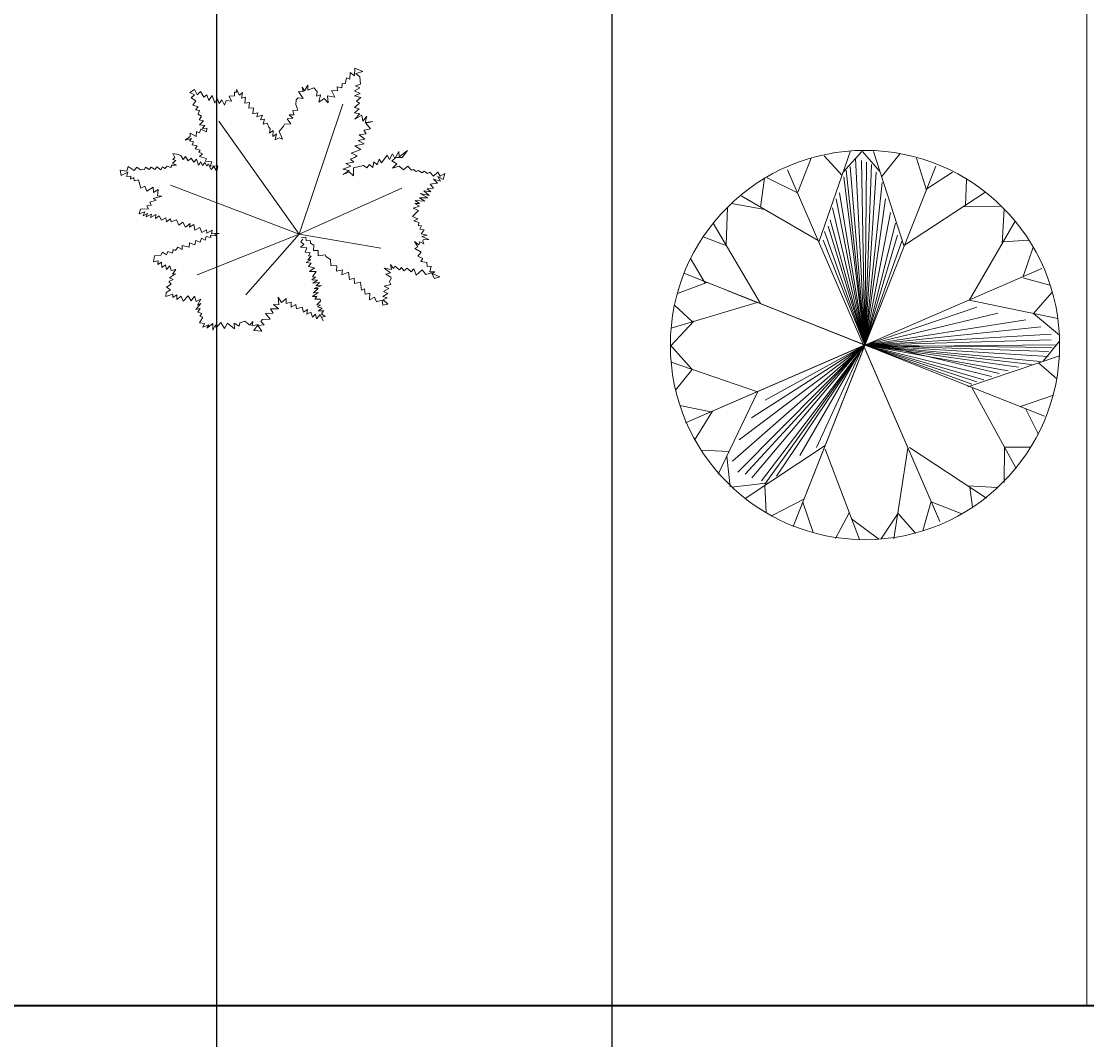
# Model space of a CAD drawing. Units: inches. Extents: x 8049 to 8459, y 820 to 1350.
# Tile 13 of 25: x 8170 to 8197, y 853 to 879. Entities that reach past the tile are written whole.
import ezdxf

# ---------------------------------------------------------------- set-up
doc = ezdxf.new("R2010")
doc.units = ezdxf.units.IN
doc.header["$MEASUREMENT"] = 0
for name, color, linetype, lineweight in [('A-ANNO-DIMS', 2, 'Continuous', 18), ('C-SITE-WALL', 7, 'Continuous', 35), ('L-PLNT-BEDS', 94, 'Continuous', 18), ('zelen', 69, 'Continuous', 13)]:
    doc.layers.add(name, color=color, linetype=linetype, lineweight=lineweight)
doc.styles.get("Standard").update_dxf_attribs({"font": 'arial.ttf'})
doc.dimstyles.get("Standard").update_dxf_attribs({"dimtxt": 0.18, "dimasz": 0.18, "dimexe": 0.18, "dimexo": 0.0625, "dimgap": 0.09, "dimtad": 0, "dimtih": 1, "dimtoh": 1, "dimdec": 4, "dimzin": 0, "dimdsep": 46, "dimtxsty": 'Standard', "dimcen": 0.09, "dimadec": 0, "dimazin": 0, "dimtfac": 1, "dimtdec": 4, "dimtofl": 0, "dimtmove": 0, "dimatfit": 3, "dimfxl": 1, "dimtolj": 1, "dimtzin": 0, "dimarcsym": 0})

# ---------------------------------------------------------------- blocks, each defined once
blk = doc.blocks.new('z_85')
for p, q in [((154.8, 474.2), (155.6, 493.8)), ((155.6, 493.8), (168.5, 483.9)), ((168.5, 483.9), (169.7, 507.5)), ((169.7, 507.5), (194.7, 497.5)), ((194.7, 497.5), (173, 491.4)), ((173, 491.4), (185.2, 481.2)), ((130, 447.6), (130.9, 460.7)), ((130.9, 460.7), (140.4, 459.9)), ((140.4, 459.9), (144.1, 478.3)), ((144.1, 478.3), (154.8, 474.2)), ((186.9, 458.5), (172.1, 453.2)), ((185.2, 481.2), (186.9, 458.5)), ((-334.5, 433), (-320.5, 441.8)), ((-320.3, 426.3), (-334.5, 433)), ((-331, 417), (-320.3, 426.3)), ((-320.5, 441.8), (-312.2, 426.3)), ((-312.2, 426.3), (-302, 436.4)), ((-302, 436.4), (-292.5, 418.9)), ((-292.5, 418.9), (-282.7, 426.1)), ((-282.7, 426.1), (-277, 408.1)), ((-198.5, 423), (-198.2, 434.1)), ((-198.2, 434.1), (-192.6, 433.8)), ((-192.6, 433.8), (-192.5, 442.2)), ((-192.5, 442.2), (-183.3, 424.5)), ((-183.3, 424.5), (-173.3, 433.2)), ((-173.3, 433.2), (-176.4, 415.5)), ((-2.1, 435.8), (11.7, 434.9)), ((11.4, 414.5), (-2.1, 435.8)), ((8.4, 449), (15.4, 438)), ((11.7, 434.9), (8.4, 449)), ((15.4, 438), (25.6, 455.6)), ((25.6, 455.6), (26.4, 439.7)), ((26.4, 439.7), (44.1, 447.4)), ((44.1, 447.4), (54.4, 436.3)), ((54.4, 436.3), (52.3, 421.7)), ((52.3, 421.7), (64.6, 426)), ((64.6, 426), (59.8, 403.9)), ((98.5, 438.8), (116.6, 438)), ((108.9, 418.4), (98.5, 438.8)), ((116.1, 450.2), (130, 447.6)), ((116.6, 438), (116.1, 450.2)), ((185.1, 447.3), (169, 438)), ((169, 438), (186.4, 430.3)), ((186.4, 430.3), (169.1, 422.7)), ((172.1, 453.2), (185.1, 447.3)), ((-316.9, 407.2), (-331, 417)), ((-325.3, 394.5), (-316.9, 407.2)), ((-309.5, 388.7), (-325.3, 394.5)), ((-277, 408.1), (-266.3, 423.5)), ((-266.3, 423.5), (-258.7, 400.7)), ((-258.7, 400.7), (-250.8, 414.2)), ((-250.8, 414.2), (-244.9, 399.8)), ((-244.9, 399.8), (-237.2, 410.8)), ((-237.2, 410.8), (-228.5, 393.9)), ((-228.5, 393.9), (-223.5, 408.6)), ((-223.5, 408.6), (-207.8, 406.4)), ((-214.2, 421.3), (-198.5, 423)), ((-207.8, 406.4), (-214.2, 421.3)), ((-176.4, 415.5), (-165.1, 418.9)), ((-165.1, 418.9), (-166.4, 400.3)), ((-166.4, 400.3), (-152.4, 402.8)), ((-152.4, 402.8), (-154.8, 385.2)), ((-10.8, 396), (-9.6, 410.9)), ((-4.1, 379.1), (-10.8, 396)), ((-9.6, 410.9), (-3.8, 416.9)), ((-3.8, 416.9), (11.4, 414.5)), ((0, 0), (132.7, 397)), ((59.8, 403.9), (75.6, 414.2)), ((75.6, 414.2), (88.3, 401.4)), ((86.4, 422.5), (108.9, 418.4)), ((88.3, 401.4), (86.4, 422.5)), ((169.1, 422.7), (188.1, 417.5)), ((183.6, 400.7), (169.1, 387.1)), ((188.1, 417.5), (174.5, 406.5)), ((174.5, 406.5), (183.6, 400.7)), ((-317.2, 380.4), (-309.5, 388.7)), ((-305.1, 378.2), (-317.2, 380.4)), ((-309.5, 366.8), (-305.1, 378.2)), ((-299.2, 360.3), (-309.5, 366.8)), ((-305.9, 349.8), (-299.2, 360.3)), ((-154.8, 385.2), (-139.8, 385.6)), ((-139.8, 385.6), (-142, 367.5)), ((-142, 367.5), (-126.8, 370.7)), ((-126.8, 370.7), (-129.7, 358.9)), ((-129.7, 358.9), (-112.6, 364.1)), ((-112.6, 364.1), (-118.7, 349.7)), ((-31.2, 364.3), (-16.4, 364.7)), ((-19.6, 354.2), (-31.2, 364.3)), ((-19.9, 378.2), (-4.1, 379.1)), ((-16.4, 364.7), (-19.9, 378.2)), ((182.7, 383.5), (168.5, 371)), ((168.5, 371), (185.5, 367.5)), ((169.1, 387.1), (182.7, 383.5)), ((185.5, 367.5), (169.7, 351.3)), ((169.7, 351.3), (191.1, 364.1)), ((191.1, 364.1), (194, 345.3)), ((194, 345.3), (206.3, 360.8)), ((206.3, 360.8), (201.7, 341.2)), ((-292.6, 345.9), (-305.9, 349.8)), ((-305.3, 333.9), (-292.6, 345.9)), ((-288.9, 332.3), (-305.3, 333.9)), ((-296.8, 323.1), (-288.9, 332.3)), ((0, 0), (-245.8, 345.3)), ((-118.7, 349.7), (-106.5, 351.7)), ((-106.5, 351.7), (-110.4, 335.8)), ((-110.4, 335.8), (-98.6, 339.2)), ((-98.6, 339.2), (-92.9, 326.8)), ((-92.9, 326.8), (-89.6, 322.3)), ((-61.6, 314), (-48.8, 329.6)), ((-48.8, 329.6), (-45, 336.2)), ((-45, 336.2), (-26.1, 337)), ((-37.5, 352.7), (-19.6, 354.2)), ((-26.1, 337), (-37.5, 352.7)), ((201.7, 341.2), (224.8, 344.2)), ((224.8, 344.2), (203.2, 339.2)), ((203.2, 339.2), (217.5, 321.8)), ((-348.8, 287.5), (-334.3, 298.5)), ((-334.3, 298.5), (-333.4, 308.7)), ((-333.4, 308.7), (-315.2, 298.3)), ((-315.2, 298.3), (-314.9, 314.1)), ((-314.9, 314.1), (-305, 309.4)), ((-305, 309.4), (-300.9, 321)), ((-300.9, 321), (-284.3, 312.7)), ((-283.1, 324), (-296.8, 323.1)), ((-284.3, 312.7), (-283.1, 324)), ((-89.6, 322.3), (-91.1, 309)), ((-91.1, 309), (-80.4, 316.3)), ((-80.4, 316.3), (-81.2, 298.5)), ((-81.2, 298.5), (-70.2, 306.6)), ((-70.2, 306.6), (-73.6, 287.8)), ((-73.6, 287.8), (-62, 294.6)), ((-62, 294.6), (-51.7, 290.2)), ((-51.7, 290.2), (-61.6, 314)), ((204.7, 306.3), (183.1, 303.2)), ((183.1, 303.2), (199.8, 290.5)), ((217.5, 321.8), (196.8, 317.3)), ((196.8, 317.3), (204.7, 306.3)), ((-329.7, 291.9), (-348.8, 287.5)), ((-335.7, 285.2), (-329.7, 291.9)), ((-323.9, 282.5), (-335.7, 285.2)), ((-327.7, 273.4), (-323.9, 282.5)), ((-312.5, 269.8), (-327.7, 273.4)), ((-318.1, 260.9), (-312.5, 269.8)), ((-303.5, 257.1), (-318.1, 260.9)), ((198, 276.2), (169.3, 269.4)), ((169.3, 269.4), (187.9, 258.2)), ((199.8, 290.5), (179.5, 286.4)), ((179.5, 286.4), (198, 276.2)), ((-387.2, 228.2), (-380.3, 234.1)), ((-377.3, 224.9), (-387.2, 228.2)), ((-386.6, 246.8), (-370.9, 243.8)), ((-380.3, 234.1), (-386.6, 246.8)), ((-370.9, 243.8), (-362.5, 240.1)), ((-362.5, 240.1), (-355.4, 227.7)), ((-355.4, 227.7), (-347.7, 237.1)), ((-347.7, 237.1), (-340.1, 223.9)), ((-340.1, 223.9), (-331.2, 232.1)), ((-331.2, 232.1), (-323, 219.9)), ((-323, 219.9), (-314.9, 229.4)), ((-314.9, 229.4), (-308.7, 210.5)), ((-306.9, 250.2), (-303.5, 257.1)), ((-296.5, 245.4), (-306.9, 250.2)), ((-304.8, 236.9), (-296.5, 245.4)), ((-284, 230.8), (-304.8, 236.9)), ((-287.5, 222.7), (-284, 230.8)), ((169.1, 234), (156.5, 228.6)), ((156.5, 228.6), (166.6, 220)), ((187.9, 258.2), (158.6, 247.3)), ((158.6, 247.3), (176.5, 239.3)), ((176.5, 239.3), (169.1, 234)), ((237.6, 211.9), (244, 229.6)), ((244, 229.6), (251.2, 218.3)), ((251.2, 218.3), (269.1, 241.8)), ((269.1, 241.8), (276.1, 228.2)), ((276.1, 228.2), (284.6, 245.4)), ((291.9, 231.3), (282.8, 224.3)), ((284.6, 245.4), (292.5, 230.8)), ((294, 233.8), (291.9, 231.3)), ((292.5, 230.8), (304.2, 252.6)), ((314, 234.4), (294, 233.8)), ((304.2, 252.6), (305.4, 235.8)), ((305.4, 235.8), (330.6, 255.3)), ((330.6, 255.3), (314, 234.4)), ((-527.9, 192.6), (-523, 206.4)), ((-523, 206.4), (-504.7, 194.2)), ((-504.7, 194.2), (-496.5, 204.8)), ((-496.5, 204.8), (-486, 196.2)), ((-486, 196.2), (-473.8, 197.3)), ((-473.8, 197.3), (-470.6, 205)), ((-470.6, 205), (-459, 197.9)), ((-459, 197.9), (-453.2, 204.7)), ((-453.2, 204.7), (-441.7, 197.3)), ((-441.7, 197.3), (-436, 206.1)), ((-436, 206.1), (-423, 196.7)), ((-423, 196.7), (-417.9, 205.5)), ((-417.9, 205.5), (-411.3, 200.8)), ((-411.3, 200.8), (-403.9, 207.3)), ((-403.9, 207.3), (-392, 203.9)), ((-392, 203.9), (-391, 210.5)), ((-391, 210.5), (-375.1, 210.9)), ((-387.5, 216.4), (-377.3, 224.9)), ((-375.1, 210.9), (-387.5, 216.4)), ((-308.7, 210.5), (-301.4, 220.5)), ((-301.4, 220.5), (-296.2, 209.5)), ((-296.2, 209.5), (-288.7, 218.5)), ((-288.7, 218.5), (-282.8, 208)), ((-267.9, 221.3), (-287.5, 222.7)), ((-282.8, 208), (-278.3, 215.3)), ((-278.3, 215.3), (-269.6, 197)), ((-272.7, 208.1), (-267.9, 221.3)), ((-249.1, 208.6), (-272.7, 208.1)), ((-269.6, 197), (-261.6, 206.7)), ((-261.6, 206.7), (-252.6, 191.1)), ((-252.6, 191.1), (-249.1, 208.6)), ((157.5, 207.7), (133, 198.3)), ((133, 198.3), (152.7, 194.8)), ((166.6, 220), (142.5, 215.8)), ((142.5, 215.8), (157.5, 207.7)), ((165.5, 178.4), (166.1, 202.2)), ((166.1, 202.2), (195.8, 210)), ((195.8, 210), (206.3, 202.3)), ((206.3, 202.3), (214.9, 212.7)), ((214.9, 212.7), (225, 203.7)), ((225, 203.7), (227.4, 221.4)), ((227.4, 221.4), (237.6, 211.9)), ((282.8, 224.3), (297.7, 215.3)), ((297.7, 215.3), (285.2, 201.4)), ((285.2, 201.4), (305.7, 207.8)), ((305.7, 207.8), (318.4, 196.7)), ((318.4, 196.7), (331.5, 207.2)), ((331.5, 207.2), (343.4, 195.3)), ((343.4, 195.3), (349.2, 197.8)), ((349.2, 197.8), (357.1, 191.7)), ((-547.4, 195.4), (-527.9, 192.6)), ((-544.7, 179.5), (-547.4, 195.4)), ((-524.7, 189.5), (-544.7, 179.5)), ((-528.5, 176.6), (-524.7, 189.5)), ((-515.5, 177.6), (-528.5, 176.6)), ((-516.7, 167.9), (-515.5, 177.6)), ((-506.3, 173.2), (-516.7, 167.9)), ((-504.7, 162.4), (-506.3, 173.2)), ((-491.4, 165.7), (-504.7, 162.4)), ((-484.9, 140.6), (-491.4, 165.7)), ((152.7, 194.8), (134.2, 181.8)), ((134.2, 181.8), (152.3, 190.3)), ((152.3, 190.3), (165.5, 178.4)), ((357.1, 191.7), (363.4, 194)), ((363.4, 194), (375.4, 187.3)), ((375.4, 187.3), (381.6, 192.9)), ((381.6, 192.9), (391.6, 185.1)), ((391.6, 185.1), (399.5, 189.8)), ((399.5, 189.8), (410.7, 177.1)), ((410.7, 177.1), (423.8, 189)), ((410.7, 167.7), (422.9, 156)), ((431.6, 161.5), (410.7, 167.7)), ((423.8, 189), (430.9, 177.3)), ((423.8, 175.6), (431.6, 161.5)), ((440.2, 166.6), (423.8, 175.6)), ((430.9, 177.3), (445.2, 185.4)), ((445.2, 185.4), (440.2, 166.6)), ((-472, 147), (-484.9, 140.6)), ((-466.4, 131.1), (-472, 147)), ((-447.4, 143.9), (-466.4, 131.1)), ((-446.4, 127.5), (-447.4, 143.9)), ((-431.2, 136.1), (-446.4, 127.5)), ((-432.5, 124.7), (-431.2, 136.1)), ((0, 0), (-394.4, 149.4)), ((0, 0), (313.9, 140.8)), ((380.7, 131.9), (397.4, 117.9)), ((402.3, 129), (380.7, 131.9)), ((410.7, 140.5), (391.1, 138)), ((391.1, 138), (402.3, 129)), ((422.9, 156), (399.8, 152.7)), ((399.8, 152.7), (410.7, 140.5)), ((-456.8, 97.3), (-437.9, 103.7)), ((-447.3, 109), (-420.9, 115.7)), ((-437.9, 103.7), (-447.3, 109)), ((-433.6, 116.8), (-432.5, 124.7)), ((-420.9, 115.7), (-433.6, 116.8)), ((354.4, 102.3), (367.3, 93.6)), ((384, 100.5), (354.4, 102.3)), ((392.9, 111.3), (367, 110.4)), ((367, 110.4), (384, 100.5)), ((370, 124.5), (392.9, 111.3)), ((397.4, 117.9), (370, 124.5)), ((-490.1, 61.5), (-485.7, 76.6)), ((-472.7, 67.7), (-490.1, 61.5)), ((-485.7, 76.6), (-461.1, 77.2)), ((-477.3, 56.2), (-472.7, 67.7)), ((-466.3, 86.6), (-452.6, 88.2)), ((-461.1, 77.2), (-466.3, 86.6)), ((-452.6, 88.2), (-456.8, 97.3)), ((367.5, 85.5), (348.2, 79.7)), ((348.2, 79.7), (364, 72.5)), ((367.3, 93.6), (352.7, 93.5)), ((352.7, 93.5), (367.5, 85.5)), ((364, 72.5), (355.3, 62.8)), ((-464.1, 63.3), (-477.3, 56.2)), ((-468.4, 52.6), (-464.1, 63.3)), ((-452, 61.1), (-468.4, 52.6)), ((-455.1, 51.2), (-452, 61.1)), ((-439, 59.8), (-455.1, 51.2)), ((-439.5, 47.5), (-439, 59.8)), ((-428.5, 56.1), (-439.5, 47.5)), ((-421.5, 42.4), (-428.5, 56.1)), ((-408.4, 49.5), (-421.5, 42.4)), ((-406.6, 37.3), (-408.4, 49.5)), ((-393.5, 46.8), (-406.6, 37.3)), ((-392.2, 37), (-393.5, 46.8)), ((-375.3, 43.4), (-392.2, 37)), ((-368.7, 27.4), (-375.3, 43.4)), ((-356.3, 36.3), (-368.7, 27.4)), ((-348.5, 20.8), (-356.3, 36.3)), ((355.3, 62.8), (346.4, 53.6)), ((346.4, 53.6), (362.3, 46.4)), ((362.3, 46.4), (350.4, 40.1)), ((350.4, 40.1), (365.4, 35.2)), ((365.4, 35.2), (364.6, 26)), ((-333.9, 32.3), (-348.5, 20.8)), ((-335.5, 21.5), (-333.9, 32.3)), ((-322.4, 29.1), (-335.5, 21.5)), ((-319.9, 12.2), (-322.4, 29.1)), ((-303.8, 20), (-319.9, 12.2)), ((0, 0), (-312.2, -125)), ((-297.7, 5.3), (-303.8, 20)), ((-284.2, 12.8), (-297.7, 5.3)), ((-282.8, 2.5), (-284.2, 12.8)), ((-266.1, 11.6), (-282.8, 2.5)), ((-268.5, 0.9), (-266.1, 11.6)), ((-245.2, 1.9), (-268.5, 0.9)), ((-258.6, 1.3), (-245.2, 1.9)), ((-256.6, -5.5), (-258.6, 1.3)), ((0, 0), (-163.1, -186)), ((0, 0), (249.7, -43.2)), ((364.6, 26), (373.9, 25.2)), ((373.9, 25.2), (368.8, 14.6)), ((368.8, 14.6), (381.5, 13.5)), ((381.5, 13.5), (372.3, 1.1)), ((372.3, 1.1), (390.8, -3.1)), ((-337, -39.8), (-335.4, -26.5)), ((-335.4, -26.5), (-320, -32.7)), ((-320, -32.7), (-316.6, -19.6)), ((-316.6, -19.6), (-303.5, -24.4)), ((-303.5, -24.4), (-299.1, -12.1)), ((-299.1, -12.1), (-288.4, -18.9)), ((-288.4, -18.9), (-284.9, -7.8)), ((-284.9, -7.8), (-270.6, -10.5)), ((-272, -3.8), (-256.6, -5.5)), ((-270.6, -10.5), (-272, -3.8)), ((14.2, -31.5), (3.8, -40.4)), ((11, -15.5), (4.4, -23.3)), ((4.4, -23.3), (14.2, -31.5)), ((19.4, -9.1), (6, -11.1)), ((20.6, -19.7), (19.4, -9.1)), ((34.5, -21), (20.6, -19.7)), ((33.9, -27.7), (34.5, -21)), ((44.7, -33.5), (33.9, -27.7)), ((352.1, -22.6), (362.5, -39.2)), ((365.2, -32.7), (352.1, -22.6)), ((368.7, -23.2), (365.2, -32.7)), ((380.7, -30.1), (368.7, -23.2)), ((390.8, -3.1), (374.2, -7.2)), ((374.2, -7.2), (396.2, -16.9)), ((378.3, -17.7), (377.9, -21.9)), ((377.9, -21.9), (380.7, -30.1)), ((396.2, -16.9), (378.3, -17.7)), ((-442.8, -66.9), (-423.6, -64.7)), ((-423.6, -64.7), (-418.1, -55.3)), ((-418.1, -55.3), (-406.6, -63.9)), ((-406.6, -63.9), (-402.1, -52.8)), ((-402.1, -52.8), (-387.5, -58.3)), ((-387.5, -58.3), (-386, -47.3)), ((-386, -47.3), (-378.3, -50.6)), ((-378.3, -50.6), (-371.8, -40.4)), ((-371.8, -40.4), (-358.3, -47.6)), ((-358.6, -35.2), (-337, -39.8)), ((-358.3, -47.6), (-358.6, -35.2)), ((3.8, -40.4), (23.3, -42)), ((23.3, -42), (17.8, -55.3)), ((17.8, -55.3), (33.3, -57.2)), ((33.3, -57.2), (27.6, -66.1)), ((43.2, -50.4), (44.7, -33.5)), ((57.8, -49.8), (43.2, -50.4)), ((57.8, -66.7), (57.8, -49.8)), ((79.4, -63.3), (57.8, -66.7)), ((80.6, -68.6), (79.4, -63.3)), ((362.5, -39.2), (352.9, -44.5)), ((352.9, -44.5), (372.4, -54.8)), ((372.4, -54.8), (362.2, -67.3)), ((-445.6, -85.2), (-442.8, -66.9)), ((-431.8, -81.7), (-445.6, -85.2)), ((-433, -93.3), (-431.8, -81.7)), ((-421.5, -86.1), (-433, -93.3)), ((-420.3, -102.3), (-421.5, -86.1)), ((-408.9, -93.6), (-420.3, -102.3)), ((-406.5, -108.7), (-408.9, -93.6)), ((-396.2, -96.8), (-406.5, -108.7)), ((-391.4, -111), (-396.2, -96.8)), ((35.4, -79.2), (20.9, -86.9)), ((20.9, -86.9), (36.1, -88.5)), ((35.8, -67.3), (26.2, -78.5)), ((26.2, -78.5), (35.4, -79.2)), ((27.6, -66.1), (35.8, -67.3)), ((36.1, -88.5), (28.2, -99.3)), ((95, -77.7), (80.6, -68.6)), ((96.5, -95.7), (95, -77.7)), ((114.9, -96.9), (96.5, -95.7)), ((113.9, -113.2), (114.9, -96.9)), ((279.1, -92.7), (281.6, -108.4)), ((288.4, -105.6), (279.1, -92.7)), ((292.3, -97.7), (288.4, -105.6)), ((306.3, -109.8), (292.3, -97.7)), ((362.2, -67.3), (377.4, -74.9)), ((377.4, -74.9), (371.4, -84.3)), ((371.4, -84.3), (390.2, -87.1)), ((390.2, -87.1), (391, -98.7)), ((391, -98.7), (403.6, -97.7)), ((403.6, -97.7), (399.4, -115.7)), ((-396.7, -133.3), (-378.8, -121.8)), ((-377.3, -108.5), (-391.4, -111)), ((-387.6, -122.5), (-377.3, -108.5)), ((-378.8, -121.8), (-387.6, -122.5)), ((28.2, -99.3), (46.8, -102.9)), ((31.9, -112.9), (31.3, -114)), ((31.3, -114), (51.4, -114.8)), ((46.8, -102.9), (31.9, -112.9)), ((51.4, -114.8), (39.8, -130.3)), ((39.8, -130.3), (49.4, -132)), ((131.6, -109.3), (113.9, -113.2)), ((129.5, -124.2), (131.6, -109.3)), ((150, -116), (129.5, -124.2)), ((153.5, -138.6), (150, -116)), ((259.9, -104.5), (278.9, -118.5)), ((281.6, -108.4), (259.9, -104.5)), ((278.9, -118.5), (264.8, -122.8)), ((264.8, -122.8), (279.4, -131.9)), ((312.3, -101.9), (306.3, -109.8)), ((319.1, -112.6), (312.3, -101.9)), ((329.4, -104.1), (319.1, -112.6)), ((341.7, -115.9), (329.4, -104.1)), ((350.6, -106.3), (341.7, -115.9)), ((357.5, -125.6), (350.6, -106.3)), ((375.9, -109.5), (357.5, -125.6)), ((386.6, -123.9), (375.9, -109.5)), ((403.8, -118.5), (386.6, -123.9)), ((399.4, -115.7), (414.2, -115.6)), ((413.1, -135.8), (403.8, -118.5)), ((414.2, -115.6), (406.2, -120.7)), ((406.2, -120.7), (430, -130.9)), ((-405.7, -161.9), (-391.7, -153.5)), ((-394, -170.7), (-405.7, -161.9)), ((-399.4, -144.9), (-386, -138.6)), ((-391.7, -153.5), (-399.4, -144.9)), ((-386, -138.6), (-396.7, -133.3)), ((49.4, -132), (38, -139.7)), ((38, -139.7), (55.7, -140.9)), ((55.7, -140.9), (40.8, -150.5)), ((40.8, -150.5), (61.7, -147.7)), ((67.9, -157.4), (45.5, -166.6)), ((61.7, -147.7), (51.2, -158.2)), ((51.2, -158.2), (67.9, -157.4)), ((168.2, -134.7), (153.5, -138.6)), ((168.7, -151.1), (168.2, -134.7)), ((187.2, -147), (168.7, -151.1)), ((190.4, -171.9), (187.2, -147)), ((279.5, -153.9), (259.5, -159.1)), ((259.5, -159.1), (273.9, -166.2)), ((280.4, -134.4), (275.3, -145.6)), ((275.3, -145.6), (279.5, -153.9)), ((279.4, -131.9), (280.4, -134.4)), ((430, -130.9), (413.1, -135.8)), ((-408.7, -191.2), (-407.1, -178.7)), ((-386.3, -183.7), (-408.7, -191.2)), ((-407.1, -178.7), (-394, -170.7)), ((-386.9, -194.2), (-386.3, -183.7)), ((-375, -185.4), (-386.9, -194.2)), ((-374.4, -200.4), (-375, -185.4)), ((-361, -190), (-374.4, -200.4)), ((-355.6, -205.5), (-361, -190)), ((-340.1, -188.9), (-355.6, -205.5)), ((-331, -204.2), (-340.1, -188.9)), ((-320.5, -190.1), (-331, -204.2)), ((-315.8, -206.4), (-320.5, -190.1)), ((-64.5, -193.4), (-63.1, -216.4)), ((-54.1, -209.7), (-64.5, -193.4)), ((57.1, -178.7), (40.5, -191.1)), ((40.5, -191.1), (53.9, -190.4)), ((57.7, -166.9), (43.5, -179.6)), ((43.5, -179.6), (57.1, -178.7)), ((45.5, -166.6), (57.7, -166.9)), ((53.9, -190.4), (47.9, -199)), ((199.5, -167.6), (190.4, -171.9)), ((201.2, -183.5), (199.5, -167.6)), ((215.4, -180.2), (201.2, -183.5)), ((214.3, -200.6), (215.4, -180.2)), ((229.7, -192.5), (214.3, -200.6)), ((235.5, -207.5), (229.7, -192.5)), ((270.6, -182.1), (255.6, -190.7)), ((255.6, -190.7), (268.7, -194.5)), ((268.7, -194.5), (256, -201.4)), ((273.9, -166.2), (257.2, -175.1)), ((257.2, -175.1), (270.6, -182.1)), ((-316.4, -230.7), (-301.2, -212.5)), ((-303, -227.7), (-316.4, -230.7)), ((-300.9, -199.4), (-315.8, -206.4)), ((-311, -217.5), (-300.9, -199.4)), ((-301.2, -212.5), (-311, -217.5)), ((-309.9, -238.3), (-303, -227.7)), ((-78.5, -215.2), (-63.4, -228.2)), ((-63.1, -216.4), (-78.5, -215.2)), ((-39.9, -196.5), (-54.1, -209.7)), ((-40.4, -212.5), (-39.9, -196.5)), ((-25.3, -207.7), (-40.4, -212.5)), ((-25.3, -223.8), (-25.3, -207.7)), ((-10.7, -215.8), (-25.3, -223.8)), ((-8.3, -228.6), (-10.7, -215.8)), ((8.9, -223.5), (-8.3, -228.6)), ((12.7, -238.7), (8.9, -223.5)), ((47.9, -199), (63.4, -198.7)), ((65.1, -205.6), (53.6, -216.1)), ((53.6, -216.1), (64.9, -216.9)), ((64.9, -216.9), (56, -222.4)), ((56, -222.4), (69.4, -226.9)), ((69.4, -226.9), (58.1, -234.3)), ((63.4, -198.7), (65.1, -205.6)), ((253.5, -202), (235.5, -207.5)), ((255.4, -217.1), (253.5, -202)), ((270.6, -214.1), (255.4, -217.1)), ((256, -201.4), (270.6, -214.1)), ((-298.3, -242.6), (-309.9, -238.3)), ((-305.3, -270.9), (-295, -254.3)), ((-304.7, -251.3), (-298.3, -242.6)), ((-295, -254.3), (-304.7, -251.3)), ((-88.9, -260), (-113.1, -261.1)), ((-79.8, -242), (-103.3, -242.6)), ((-103.3, -242.6), (-88.9, -260)), ((-63.4, -228.2), (-87.9, -229.1)), ((-87.9, -229.1), (-79.8, -242)), ((24.7, -230.5), (12.7, -238.7)), ((23, -244.8), (24.7, -230.5)), ((35.5, -238.8), (23, -244.8)), ((40.7, -254.5), (35.5, -238.8)), ((49.8, -244.9), (40.7, -254.5)), ((52.7, -259.2), (49.8, -244.9)), ((63.6, -245.9), (52.7, -259.2)), ((58.1, -234.3), (70.9, -234.4)), ((72.4, -265), (63.6, -245.9)), ((73.9, -233.5), (67.9, -243.4)), ((67.9, -243.4), (79.4, -252.4)), ((79.4, -252.4), (68.2, -253.9)), ((68.2, -253.9), (72.4, -265)), ((70.9, -234.4), (73.9, -233.5)), ((-290.1, -273.1), (-305.3, -270.9)), ((-294.6, -284.2), (-290.1, -273.1)), ((-277.1, -277.7), (-294.6, -284.2)), ((-264.9, -273), (-283.1, -288.1)), ((-283.1, -288.1), (-277.1, -277.7)), ((-264.3, -294.3), (-264.9, -273)), ((-256.6, -277.5), (-264.3, -294.3)), ((-254.5, -286.6), (-256.6, -277.5)), ((-239.6, -270.1), (-254.5, -286.6)), ((-228.6, -289.1), (-239.6, -270.1)), ((-220, -272), (-228.6, -289.1)), ((-197.9, -289.9), (-220, -272)), ((-199.2, -272), (-197.9, -289.9)), ((-184.2, -282), (-199.2, -272)), ((-182.4, -271.4), (-184.2, -282)), ((-166.3, -266.5), (-182.4, -271.4)), ((-151.2, -278.6), (-166.3, -266.5)), ((-142.3, -267.5), (-151.2, -278.6)), ((-144.6, -280.3), (-142.3, -267.5)), ((-126.2, -276.2), (-144.6, -280.3)), ((-138.9, -294.9), (-126.2, -276.2)), ((-107.8, -278), (-127.3, -279.2)), ((-127.3, -279.2), (-114.3, -296.8)), ((-113.1, -261.1), (-117.3, -267.5)), ((-117.3, -267.5), (-107.8, -278)), ((-114.3, -296.8), (-138.9, -294.9))]:
    blk.add_line(p, q)
blk = doc.blocks.new('T40C')
for p, q in [((-0.1219, 0.4263), (-0.1133, 0.5002)), ((-0.0016, 0.4444), (-0.055, 0.5069)), ((-0.0016, 0.0138), (-0.0016, 0.5115)), ((-0.0016, 0.5115), (-0.0016, -0.4769)), ((-0.0016, 0.4364), (0.0585, 0.5048)), ((-0.0016, 0.2889), (0.1386, 0.4896)), ((0.1041, 0.4402), (0.0754, 0.5038)), ((-0.0047, 0.2984), (-0.1711, 0.4799)), ((0.0979, 0.4313), (0.1806, 0.4751)), ((0.2217, 0.4068), (0.1848, 0.4759)), ((-0.2, 0.2178), (-0.2513, 0.4459)), ((-0.2374, 0.3843), (-0.221, 0.4586)), ((-0.1327, 0.438), (-0.2166, 0.4607)), ((-0.0016, 0.0138), (0.1054, 0.4378)), ((0.0011, 0.0164), (0.1417, 0.4349)), ((0.2091, 0.2244), (0.2252, 0.4573)), ((-0.2369, 0.3817), (-0.2976, 0.4118)), ((-0.0016, 0.0138), (0.1166, 0.4328)), ((-0.0016, 0.0138), (0.2033, 0.4135)), ((-0.0016, 0.0138), (0.0852, 0.4075)), ((0.0011, 0.0164), (0.1801, 0.4343)), ((0.0011, 0.0164), (0.161, 0.432)), ((0.2208, 0.3933), (0.2879, 0.4166)), ((-0.3045, 0.3219), (-0.313, 0.3998)), ((0.2979, 0.3132), (0.3134, 0.399)), ((0.3508, 0.3661), (-0.3487, -0.3333)), ((0.0011, 0.0164), (-0.3443, 0.3618)), ((-0.3443, 0.3618), (0.3464, -0.329)), ((-0.0016, 0.0138), (0.2072, 0.3567)), ((0.0011, 0.0164), (0.3508, 0.3661)), ((0.0011, 0.0164), (0.0491, 0.3369)), ((0.3008, 0.3162), (0.3801, 0.3306)), ((-0.3055, 0.3229), (-0.3893, 0.3231)), ((0.0011, 0.0164), (0.0175, 0.3021)), ((-0.3838, 0.2523), (-0.4084, 0.2975)), ((-0.0016, 0.0138), (0.1989, 0.2926)), ((0.3847, 0.2335), (0.4047, 0.2984)), ((-0.377, 0.2509), (-0.4492, 0.2275)), ((-0.2034, 0.2144), (-0.4335, 0.2627)), ((-0.0016, 0.0138), (0.1836, 0.2378)), ((0.2092, 0.2254), (0.4418, 0.2362)), ((0.3861, 0.2336), (0.4597, 0.1963)), ((0.3915, 0.2339), (0.3982, 0.2342)), ((-0.4278, 0.1246), (-0.4601, 0.209)), ((0.4263, 0.1181), (0.4586, 0.1989)), ((-0.2946, 0.0138), (-0.4744, 0.1635)), ((0.2937, 0.0138), (0.4738, 0.1555)), ((-0.4281, 0.1249), (-0.4899, 0.1006)), ((0.4291, 0.1204), (0.4873, 0.0978)), ((-0.4418, 0.0138), (-0.4967, 0.0634)), ((0.4315, 0.0138), (0.491, 0.0679)), ((-0.4277, 0.0138), (-0.4952, -0.0443)), ((0.4953, 0.0138), (-0.4939, 0.0138)), ((-0.2846, 0.0167), (-0.4721, -0.1432)), ((-0.0016, 0.0138), (-0.4477, -0.1559)), ((-0.0016, 0.0138), (-0.4464, -0.1312)), ((-0.0016, 0.0138), (-0.4422, -0.1429)), ((-0.0016, 0.0138), (-0.4379, -0.1735)), ((-0.0016, 0.0138), (-0.4328, -0.1117)), ((-0.0016, 0.0138), (-0.4324, -0.1862)), ((-0.4324, -0.1862), (-0.0016, 0.0138)), ((-0.0016, 0.0138), (-0.4146, -0.0968)), ((-0.0016, 0.0138), (-0.4013, -0.1946)), ((-0.0016, 0.0138), (-0.3864, -0.0775)), ((-0.0016, 0.0138), (-0.3647, -0.0593)), ((-0.0016, 0.0138), (-0.3588, -0.1967)), ((-0.0016, 0.0138), (-0.3309, -0.0302)), ((-0.0016, 0.0138), (-0.3156, -0.0151)), ((-0.0016, 0.0138), (-0.3007, -0.0042)), ((-0.0016, 0.0138), (-0.2917, 0.0059)), ((-0.0016, 0.0138), (-0.2861, -0.1863)), ((-0.0016, 0.0138), (-0.2311, -0.181)), ((-0.0016, 0.0138), (-0.0528, -0.0021)), ((-0.0016, 0.0138), (-0.0528, -0.0021)), ((-0.0016, 0.0138), (0.0011, 0.0164)), ((-0.0016, 0.0138), (0.4953, 0.0138)), ((-0.0016, 0.0138), (0.0088, -0.2669)), ((-0.0016, 0.0138), (0.0243, -0.2768)), ((-0.0016, 0.0138), (0.0408, -0.3033)), ((-0.0016, 0.0138), (0.0625, -0.3241)), ((-0.0016, 0.0138), (0.0872, -0.3518)), ((-0.0016, 0.0138), (0.1104, -0.3878)), ((-0.0016, 0.0138), (0.1339, -0.4064)), ((-0.0016, 0.0138), (0.1521, -0.4202)), ((-0.0016, 0.0138), (0.1669, -0.4211)), ((-0.0016, 0.0138), (0.1801, -0.4202)), ((-0.0016, 0.0138), (0.1959, -0.4202)), ((-0.0016, 0.0138), (0.2013, -0.3955)), ((-0.0016, 0.0138), (0.2072, -0.3832)), ((-0.0016, 0.0138), (0.2062, -0.3647)), ((-0.0016, 0.0138), (0.2018, -0.3233)), ((-0.0016, 0.0138), (0.2038, -0.3052)), ((-0.0016, 0.0138), (0.2044, -0.2809)), ((-0.0016, 0.0138), (0.1983, -0.2504)), ((-0.0016, 0.0138), (0.197, -0.2334)), ((-0.0016, 0.0138), (0.2007, -0.2173)), ((-0.0016, 0.0138), (0.1959, -0.1959)), ((0.285, 0.0138), (0.4722, -0.133)), ((0.2917, 0.0138), (0.3747, 0.0138)), ((0.4349, 0.0169), (0.4927, -0.0276)), ((-0.0528, -0.0021), (-0.4551, -0.1664)), ((-0.0528, -0.0021), (-0.3463, -0.045)), ((-0.4294, -0.1068), (-0.4874, -0.0863)), ((0.4191, -0.0914), (0.4833, -0.0909)), ((0.4217, -0.0934), (0.4533, -0.184)), ((-0.4387, -0.1147), (-0.459, -0.1779)), ((0.2042, -0.1867), (0.2149, -0.4325)), ((0.2071, -0.1897), (0.4318, -0.2236)), ((-0.3712, -0.2192), (-0.4529, -0.1923)), ((-0.2066, -0.1906), (-0.4335, -0.23)), ((-0.2067, -0.1914), (-0.2414, -0.4204)), ((0.3628, -0.2132), (0.4476, -0.1967)), ((0.3755, -0.2151), (0.3928, -0.2871)), ((-0.3712, -0.2192), (-0.3953, -0.2872)), ((-0.0016, -0.2596), (-0.1424, -0.4599)), ((-0.0016, -0.2565), (0.16, -0.4525)), ((-0.3126, -0.2938), (-0.3837, -0.3016)), ((-0.3124, -0.2971), (-0.3082, -0.3761)), ((0.3007, -0.2833), (0.3874, -0.2905)), ((0.3008, -0.2851), (0.3017, -0.3787)), ((-0.2322, -0.3601), (-0.2902, -0.3882)), ((-0.2315, -0.3548), (-0.2033, -0.4394)), ((0.2123, -0.3741), (0.1875, -0.442)), ((0.212, -0.3667), (0.2724, -0.3967)), ((-0.1046, -0.4061), (-0.1917, -0.4425)), ((0.1172, -0.4006), (0.0947, -0.4728)), ((-0.1086, -0.4118), (-0.0869, -0.4727)), ((-0.0016, -0.4144), (-0.047, -0.4779)), ((-0.0016, -0.4109), (0.0515, -0.477)), ((0.1259, -0.4112), (0.1857, -0.4428))]:
    blk.add_line(p, q)
blk.add_circle((-0.0016, 0.0138), 0.496)
blk = doc.blocks.new('*D58')
at = {"layer": 'A-ANNO-DIMS', "color": 0, "lineweight": -2, "transparency": 16777216}
for p, q in [((8139.397, 1162.808), (8139.397, 820.091)), ((8175.397, 1162.808), (8175.397, 820.091)), ((8139.577, 820.271), (8157.179, 820.271)), ((8175.217, 820.271), (8157.616, 820.271))]:
    blk.add_line(p, q, dxfattribs=at)
at = {"layer": 'A-ANNO-DIMS', "color": 0, "transparency": 16777216}
for points in [[(8139.577, 820.301), (8139.577, 820.241), (8139.397, 820.271)], [(8175.217, 820.301), (8175.217, 820.241), (8175.397, 820.271)]]:
    blk.add_solid(points, dxfattribs=at)
at = {"layer": 'Defpoints', "color": 0, "transparency": 16777216}
for p in [(8139.397, 1162.871), (8175.397, 1162.871), (8175.397, 820.271)]:
    blk.add_point(p, dxfattribs=at)
at = {"layer": 'A-ANNO-DIMS', "color": 0, "transparency": 16777216, "insert": (8157.397, 820.271), "char_height": 0.18, "attachment_point": 5}
blk.add_mtext('\\A1;36', dxfattribs=at)
blk = doc.blocks.new('*D71')
at = {"layer": 'A-ANNO-DIMS', "color": 0, "lineweight": -2, "transparency": 16777216}
for p, q in [((8185.397, 1045.808), (8185.397, 820.091)), ((8239.397, 1045.808), (8239.397, 820.091)), ((8185.577, 820.271), (8212.179, 820.271)), ((8239.217, 820.271), (8212.616, 820.271))]:
    blk.add_line(p, q, dxfattribs=at)
at = {"layer": 'A-ANNO-DIMS', "color": 0, "transparency": 16777216}
for points in [[(8185.577, 820.301), (8185.577, 820.241), (8185.397, 820.271)], [(8239.217, 820.301), (8239.217, 820.241), (8239.397, 820.271)]]:
    blk.add_solid(points, dxfattribs=at)
at = {"layer": 'Defpoints', "color": 0, "transparency": 16777216}
for p in [(8185.397, 1045.871), (8239.397, 1045.871), (8239.397, 820.271)]:
    blk.add_point(p, dxfattribs=at)
at = {"layer": 'A-ANNO-DIMS', "color": 0, "transparency": 16777216, "insert": (8212.397, 820.271), "char_height": 0.18, "attachment_point": 5}
blk.add_mtext('\\A1;54', dxfattribs=at)
blk = doc.blocks.new('*D76')
at = {"layer": 'A-ANNO-DIMS', "color": 0, "lineweight": -2, "transparency": 16777216}
for p, q in [((8083.397, 1054.808), (8083.397, 820.091)), ((8299.397, 1054.808), (8299.397, 820.091)), ((8083.577, 820.271), (8191.107, 820.271)), ((8299.217, 820.271), (8191.688, 820.271))]:
    blk.add_line(p, q, dxfattribs=at)
at = {"layer": 'A-ANNO-DIMS', "color": 0, "transparency": 16777216}
for points in [[(8083.577, 820.301), (8083.577, 820.241), (8083.397, 820.271)], [(8299.217, 820.301), (8299.217, 820.241), (8299.397, 820.271)]]:
    blk.add_solid(points, dxfattribs=at)
at = {"layer": 'Defpoints', "color": 0, "transparency": 16777216}
for p in [(8083.397, 1054.871), (8299.397, 1054.871), (8299.397, 820.271)]:
    blk.add_point(p, dxfattribs=at)
at = {"layer": 'A-ANNO-DIMS', "color": 0, "transparency": 16777216, "insert": (8191.397, 820.271), "char_height": 0.18, "attachment_point": 5}
blk.add_mtext('\\A1;216', dxfattribs=at)

msp = doc.modelspace()

# ---------------------------------------------------------------- linework, layer by layer
at = {"layer": 'C-SITE-WALL'}
msp.add_line((8083.3974, 853.8706), (8219.8974, 853.8706), dxfattribs=at)
at = {"layer": 'L-PLNT-BEDS'}
msp.add_line((8197.3974, 949.8706), (8197.3974, 853.8706), dxfattribs=at)

# ---------------------------------------------------------------- block references
at = {"layer": 'zelen', "xscale": 0.0082668533249786, "yscale": 0.0082668533249786, "zscale": 0.0082668533249786}
msp.add_blockref('z_85', (8177.4938, 873.3752), dxfattribs=at)
at = {"layer": 'zelen', "xscale": 9.920223989974332, "yscale": 9.920223989974332, "zscale": 9.920223989974332, "rotation": 158.4000000000004}
msp.add_blockref('T40C', (8191.8288, 870.7033), dxfattribs=at)

# ---------------------------------------------------------------- dimensions: what is measured, and where the dimension line sits
at = {"layer": 'A-ANNO-DIMS'}
for base, p1, p2, picture, middle in [((8175.3974, 820.2706), (8139.3974, 1162.8706), (8175.3974, 1162.8706), '*D58', (8157.3974, 820.2706)), ((8299.3974, 820.2706), (8083.3974, 1054.8706), (8299.3974, 1054.8706), '*D76', (8191.3974, 820.2706)), ((8239.3974, 820.2706), (8185.3974, 1045.8706), (8239.3974, 1045.8706), '*D71', (8212.3974, 820.2706))]:
    dim = msp.add_linear_dim(base=base, p1=p1, p2=p2, dimstyle='Standard', override={"dimdec": 0, "dimlfac": 1, "dimrnd": 0, "dimzin": 0, "dimdsep": 46, "dimlunit": 2}, dxfattribs=at)
    dim.commit()
    dim.dimension.update_dxf_attribs({"geometry": picture, "text_midpoint": middle})

doc.saveas('drawing.dxf')
